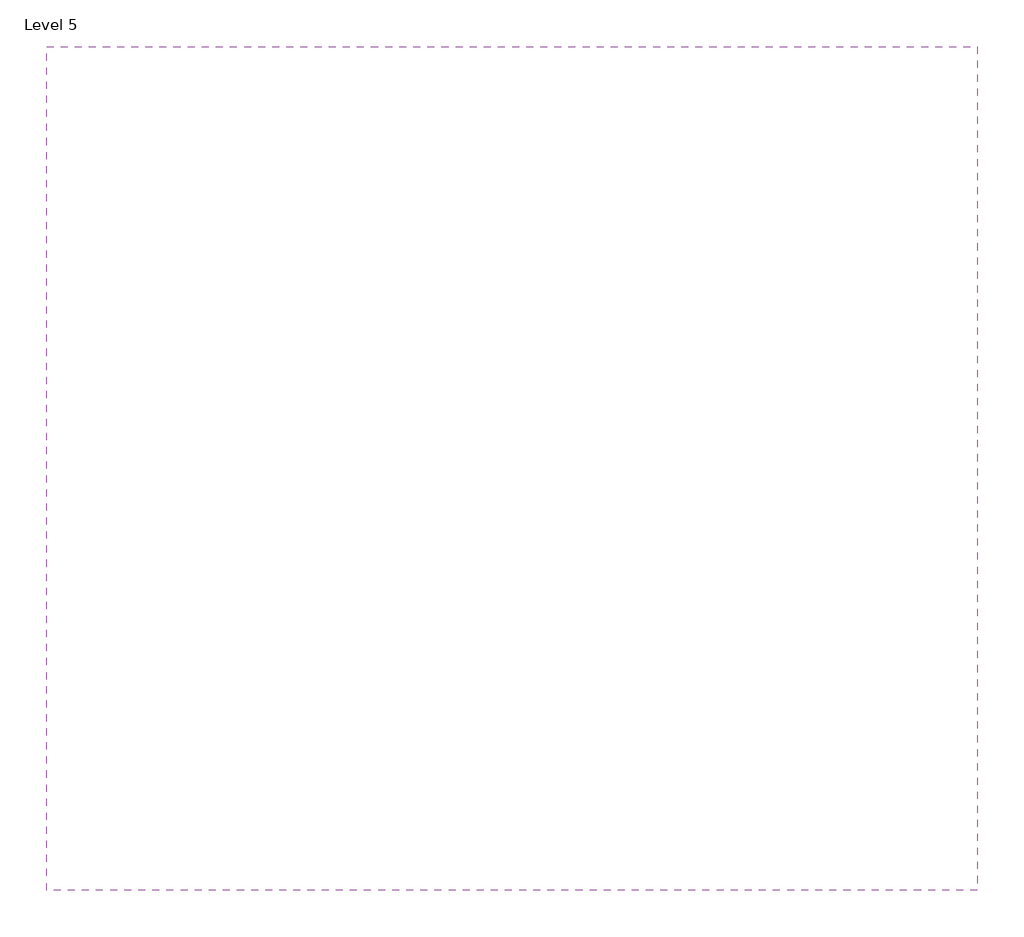
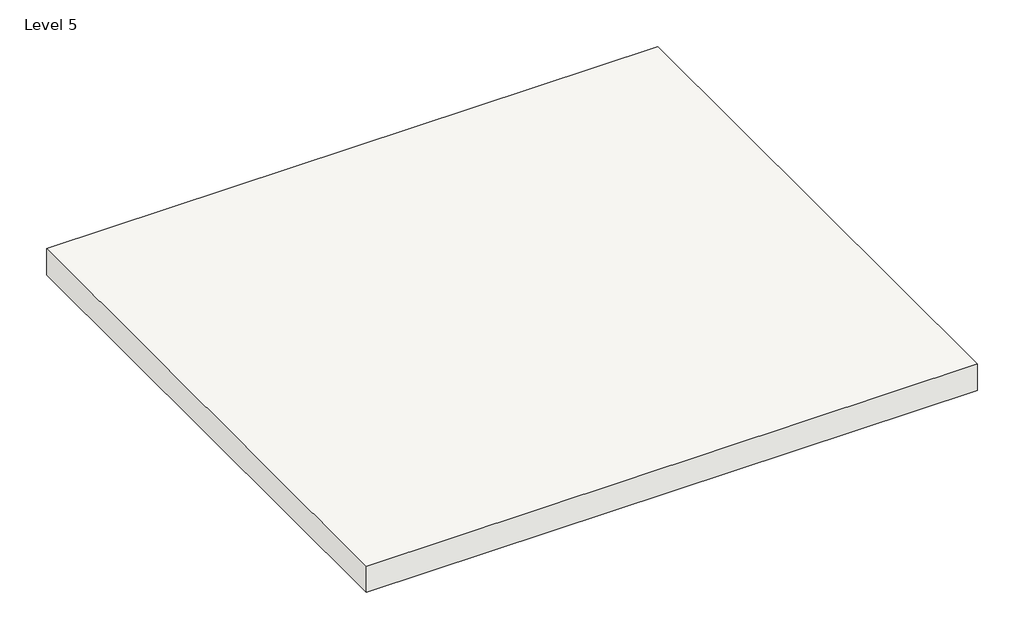
# One storey: 1 slab.
"""IFC4 building model written with IfcOpenShell, lengths in millimetres."""

from ifc_helpers import new_model, si_unit, frame, origin, place, context, project, spatial, polyline, outline, extrude, element, save

model = new_model("IFC4")

# Units and contexts
model_context = context("Model", 3, world=origin())
ifc_project = project(units=[si_unit("LENGTHUNIT", "METRE", prefix="MILLI")], contexts=[model_context])

# Site, building, storey
site = spatial("IfcSite", under=ifc_project)
building = spatial("IfcBuilding", under=site)
storey = spatial("IfcBuildingStorey", under=building, Name="Level 5", Elevation=7620.0)

# Slab
placement = place(None, origin())
element("IfcSlab", 1, ObjectType="SLAB 6\"", at=placement, inside=storey, context=model_context, shape_type="SweptSolid", body=[
    extrude(outline(polyline([(-6247.3892099, 69.3888401), (-9609.3179063, 69.3888401), (-9609.3179063, 3117.3888401), (-6247.3892099, 3117.3888401), (-6247.3892099, 69.3888401)])), frame((0.0, 0.0, 9601.2), z_axis=(0.0, 0.0, 1.0), x_axis=(1.0, 0.0, 0.0)), (0.0, 0.0, 1.0), 152.4),
])

save(model, "model.ifc")

# Revit data of these elements
# Type "SLAB 6\""
#   Assembly Code = "B1010"
#   Function = 0
#   Layers, outside or top first: 0' - 6" no material (function 1)
# Element 1 (IfcSlab, "SLAB 6\"")
#   Height Offset From Level = 7' - 0"
#   Phase Created = New Construction
#   Materials on its faces: "Default Floor"
# Materials
#   "Default Floor": colour RGB 128 128 128, transparency 0, Cost = 0
